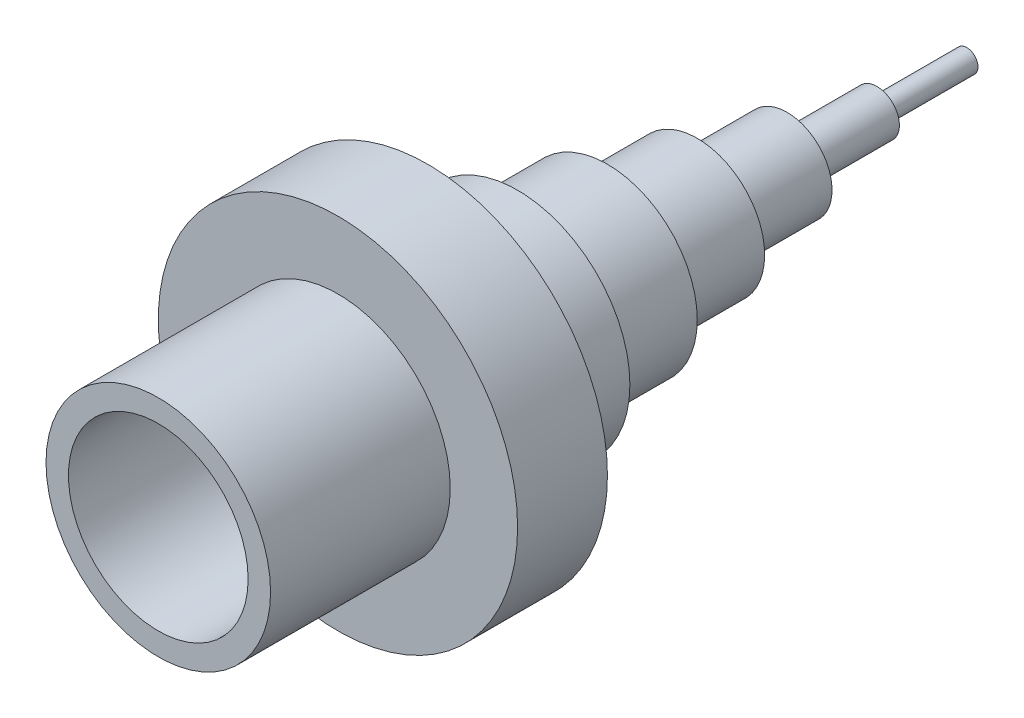
ISO-10303-21;
HEADER;
FILE_DESCRIPTION(('STEP AP214'),'2;1');
FILE_NAME('part.step','',(''),(''),'','','');
FILE_SCHEMA(('AUTOMOTIVE_DESIGN { 1 0 10303 214 1 1 1 1 }'));
ENDSEC;
DATA;
#1=APPLICATION_CONTEXT('core data for automotive mechanical design processes');
#2=APPLICATION_PROTOCOL_DEFINITION('international standard','automotive_design',2000,#1);
#3=PRODUCT_CONTEXT('',#1,'mechanical');
#4=PRODUCT('Part','Part','',(#3));
#5=PRODUCT_RELATED_PRODUCT_CATEGORY('part','',(#4));
#6=PRODUCT_DEFINITION_FORMATION('','',#4);
#7=PRODUCT_DEFINITION_CONTEXT('part definition',#1,'design');
#8=PRODUCT_DEFINITION('design','',#6,#7);
#9=PRODUCT_DEFINITION_SHAPE('','',#8);
#10=(LENGTH_UNIT() NAMED_UNIT(*) SI_UNIT(.MILLI.,.METRE.));
#11=(NAMED_UNIT(*) PLANE_ANGLE_UNIT() SI_UNIT($,.RADIAN.));
#12=(NAMED_UNIT(*) SI_UNIT($,.STERADIAN.) SOLID_ANGLE_UNIT());
#13=UNCERTAINTY_MEASURE_WITH_UNIT(LENGTH_MEASURE(1.E-05),#10,'distance_accuracy_value','');
#14=(GEOMETRIC_REPRESENTATION_CONTEXT(3) GLOBAL_UNCERTAINTY_ASSIGNED_CONTEXT((#13)) GLOBAL_UNIT_ASSIGNED_CONTEXT((#10,
#11,#12)) REPRESENTATION_CONTEXT('',''));
#15=CARTESIAN_POINT('',(0.,0.,0.));
#16=DIRECTION('',(0.,0.,1.));
#17=DIRECTION('',(1.,0.,0.));
#18=AXIS2_PLACEMENT_3D('',#15,#16,#17);
#19=CARTESIAN_POINT('',(0.,0.,-20.));
#20=DIRECTION('',(0.,0.,1.));
#21=DIRECTION('',(1.,0.,0.));
#22=AXIS2_PLACEMENT_3D('',#19,#20,#21);
#23=CYLINDRICAL_SURFACE('',#22,40.);
#24=CARTESIAN_POINT('',(0.,0.,-20.));
#25=DIRECTION('',(0.,0.,1.));
#26=DIRECTION('',(1.,0.,0.));
#27=AXIS2_PLACEMENT_3D('',#24,#25,#26);
#28=CIRCLE('',#27,40.);
#29=CARTESIAN_POINT('',(40.,0.,-20.));
#30=VERTEX_POINT('',#29);
#31=EDGE_CURVE('E42',#30,#30,#28,.T.);
#32=ORIENTED_EDGE('',*,*,#31,.T.);
#33=EDGE_LOOP('',(#32));
#34=FACE_BOUND('',#33,.T.);
#35=CARTESIAN_POINT('',(0.,0.,0.));
#36=DIRECTION('',(0.,0.,1.));
#37=DIRECTION('',(1.,0.,0.));
#38=AXIS2_PLACEMENT_3D('',#35,#36,#37);
#39=CIRCLE('',#38,40.);
#40=CARTESIAN_POINT('',(40.,0.,0.));
#41=VERTEX_POINT('',#40);
#42=EDGE_CURVE('E47',#41,#41,#39,.T.);
#43=ORIENTED_EDGE('',*,*,#42,.F.);
#44=EDGE_LOOP('',(#43));
#45=FACE_BOUND('',#44,.T.);
#46=ADVANCED_FACE('F40',(#34,#45),#23,.T.);
#47=CARTESIAN_POINT('',(0.,0.,-20.));
#48=DIRECTION('',(0.,0.,1.));
#49=DIRECTION('',(1.,0.,0.));
#50=AXIS2_PLACEMENT_3D('',#47,#48,#49);
#51=PLANE('',#50);
#52=CARTESIAN_POINT('',(0.,0.,-20.));
#53=DIRECTION('',(0.,0.,1.));
#54=DIRECTION('',(1.,0.,0.));
#55=AXIS2_PLACEMENT_3D('',#52,#53,#54);
#56=CIRCLE('',#55,25.);
#57=CARTESIAN_POINT('',(25.,0.,-20.));
#58=VERTEX_POINT('',#57);
#59=EDGE_CURVE('E80',#58,#58,#56,.T.);
#60=ORIENTED_EDGE('',*,*,#59,.T.);
#61=EDGE_LOOP('',(#60));
#62=FACE_BOUND('',#61,.T.);
#63=ORIENTED_EDGE('',*,*,#31,.F.);
#64=EDGE_LOOP('',(#63));
#65=FACE_BOUND('',#64,.T.);
#66=ADVANCED_FACE('F108',(#62,#65),#51,.F.);
#67=CARTESIAN_POINT('',(0.,0.,0.));
#68=DIRECTION('',(0.,0.,1.));
#69=DIRECTION('',(1.,0.,0.));
#70=AXIS2_PLACEMENT_3D('',#67,#68,#69);
#71=PLANE('',#70);
#72=CARTESIAN_POINT('',(0.,0.,0.));
#73=DIRECTION('',(0.,0.,1.));
#74=DIRECTION('',(1.,0.,0.));
#75=AXIS2_PLACEMENT_3D('',#72,#73,#74);
#76=CIRCLE('',#75,25.);
#77=CARTESIAN_POINT('',(25.,0.,0.));
#78=VERTEX_POINT('',#77);
#79=EDGE_CURVE('E10',#78,#78,#76,.T.);
#80=ORIENTED_EDGE('',*,*,#79,.F.);
#81=EDGE_LOOP('',(#80));
#82=FACE_BOUND('',#81,.T.);
#83=ORIENTED_EDGE('',*,*,#42,.T.);
#84=EDGE_LOOP('',(#83));
#85=FACE_BOUND('',#84,.T.);
#86=ADVANCED_FACE('F113',(#82,#85),#71,.T.);
#87=CARTESIAN_POINT('',(0.,0.,-40.));
#88=DIRECTION('',(0.,0.,1.));
#89=DIRECTION('',(1.,0.,0.));
#90=AXIS2_PLACEMENT_3D('',#87,#88,#89);
#91=CYLINDRICAL_SURFACE('',#90,25.);
#92=CARTESIAN_POINT('',(0.,0.,-40.));
#93=DIRECTION('',(0.,0.,1.));
#94=DIRECTION('',(1.,0.,0.));
#95=AXIS2_PLACEMENT_3D('',#92,#93,#94);
#96=CIRCLE('',#95,25.);
#97=CARTESIAN_POINT('',(25.,0.,-40.));
#98=VERTEX_POINT('',#97);
#99=EDGE_CURVE('E73',#98,#98,#96,.T.);
#100=ORIENTED_EDGE('',*,*,#99,.T.);
#101=EDGE_LOOP('',(#100));
#102=FACE_BOUND('',#101,.T.);
#103=ORIENTED_EDGE('',*,*,#59,.F.);
#104=EDGE_LOOP('',(#103));
#105=FACE_BOUND('',#104,.T.);
#106=ADVANCED_FACE('F122',(#102,#105),#91,.T.);
#107=CARTESIAN_POINT('',(0.,0.,-40.));
#108=DIRECTION('',(0.,0.,1.));
#109=DIRECTION('',(1.,0.,0.));
#110=AXIS2_PLACEMENT_3D('',#107,#108,#109);
#111=PLANE('',#110);
#112=CARTESIAN_POINT('',(0.,0.,-40.));
#113=DIRECTION('',(0.,0.,1.));
#114=DIRECTION('',(1.,0.,0.));
#115=AXIS2_PLACEMENT_3D('',#112,#113,#114);
#116=CIRCLE('',#115,20.);
#117=CARTESIAN_POINT('',(20.,0.,-40.));
#118=VERTEX_POINT('',#117);
#119=EDGE_CURVE('E75',#118,#118,#116,.T.);
#120=ORIENTED_EDGE('',*,*,#119,.T.);
#121=EDGE_LOOP('',(#120));
#122=FACE_BOUND('',#121,.T.);
#123=ORIENTED_EDGE('',*,*,#99,.F.);
#124=EDGE_LOOP('',(#123));
#125=FACE_BOUND('',#124,.T.);
#126=ADVANCED_FACE('F130',(#122,#125),#111,.F.);
#127=CARTESIAN_POINT('',(0.,0.,-60.));
#128=DIRECTION('',(0.,0.,1.));
#129=DIRECTION('',(1.,0.,0.));
#130=AXIS2_PLACEMENT_3D('',#127,#128,#129);
#131=CYLINDRICAL_SURFACE('',#130,20.);
#132=CARTESIAN_POINT('',(0.,0.,-60.));
#133=DIRECTION('',(0.,0.,1.));
#134=DIRECTION('',(1.,0.,0.));
#135=AXIS2_PLACEMENT_3D('',#132,#133,#134);
#136=CIRCLE('',#135,20.);
#137=CARTESIAN_POINT('',(20.,0.,-60.));
#138=VERTEX_POINT('',#137);
#139=EDGE_CURVE('E69',#138,#138,#136,.T.);
#140=ORIENTED_EDGE('',*,*,#139,.T.);
#141=EDGE_LOOP('',(#140));
#142=FACE_BOUND('',#141,.T.);
#143=ORIENTED_EDGE('',*,*,#119,.F.);
#144=EDGE_LOOP('',(#143));
#145=FACE_BOUND('',#144,.T.);
#146=ADVANCED_FACE('F132',(#142,#145),#131,.T.);
#147=CARTESIAN_POINT('',(0.,0.,-60.));
#148=DIRECTION('',(0.,0.,1.));
#149=DIRECTION('',(1.,0.,0.));
#150=AXIS2_PLACEMENT_3D('',#147,#148,#149);
#151=PLANE('',#150);
#152=CARTESIAN_POINT('',(0.,0.,-60.));
#153=DIRECTION('',(0.,0.,1.));
#154=DIRECTION('',(1.,0.,0.));
#155=AXIS2_PLACEMENT_3D('',#152,#153,#154);
#156=CIRCLE('',#155,15.);
#157=CARTESIAN_POINT('',(15.,0.,-60.));
#158=VERTEX_POINT('',#157);
#159=EDGE_CURVE('E67',#158,#158,#156,.T.);
#160=ORIENTED_EDGE('',*,*,#159,.T.);
#161=EDGE_LOOP('',(#160));
#162=FACE_BOUND('',#161,.T.);
#163=ORIENTED_EDGE('',*,*,#139,.F.);
#164=EDGE_LOOP('',(#163));
#165=FACE_BOUND('',#164,.T.);
#166=ADVANCED_FACE('F140',(#162,#165),#151,.F.);
#167=CARTESIAN_POINT('',(0.,0.,-80.));
#168=DIRECTION('',(0.,0.,1.));
#169=DIRECTION('',(1.,0.,0.));
#170=AXIS2_PLACEMENT_3D('',#167,#168,#169);
#171=CYLINDRICAL_SURFACE('',#170,15.);
#172=CARTESIAN_POINT('',(0.,0.,-80.));
#173=DIRECTION('',(0.,0.,1.));
#174=DIRECTION('',(1.,0.,0.));
#175=AXIS2_PLACEMENT_3D('',#172,#173,#174);
#176=CIRCLE('',#175,15.);
#177=CARTESIAN_POINT('',(15.,0.,-80.));
#178=VERTEX_POINT('',#177);
#179=EDGE_CURVE('E68',#178,#178,#176,.T.);
#180=ORIENTED_EDGE('',*,*,#179,.T.);
#181=EDGE_LOOP('',(#180));
#182=FACE_BOUND('',#181,.T.);
#183=ORIENTED_EDGE('',*,*,#159,.F.);
#184=EDGE_LOOP('',(#183));
#185=FACE_BOUND('',#184,.T.);
#186=ADVANCED_FACE('F145',(#182,#185),#171,.T.);
#187=CARTESIAN_POINT('',(0.,0.,-80.));
#188=DIRECTION('',(0.,0.,1.));
#189=DIRECTION('',(1.,0.,0.));
#190=AXIS2_PLACEMENT_3D('',#187,#188,#189);
#191=PLANE('',#190);
#192=CARTESIAN_POINT('',(0.,0.,-80.));
#193=DIRECTION('',(0.,0.,1.));
#194=DIRECTION('',(1.,0.,0.));
#195=AXIS2_PLACEMENT_3D('',#192,#193,#194);
#196=CIRCLE('',#195,10.);
#197=CARTESIAN_POINT('',(10.,0.,-80.));
#198=VERTEX_POINT('',#197);
#199=EDGE_CURVE('E62',#198,#198,#196,.T.);
#200=ORIENTED_EDGE('',*,*,#199,.T.);
#201=EDGE_LOOP('',(#200));
#202=FACE_BOUND('',#201,.T.);
#203=ORIENTED_EDGE('',*,*,#179,.F.);
#204=EDGE_LOOP('',(#203));
#205=FACE_BOUND('',#204,.T.);
#206=ADVANCED_FACE('F149',(#202,#205),#191,.F.);
#207=CARTESIAN_POINT('',(0.,0.,-100.));
#208=DIRECTION('',(0.,0.,1.));
#209=DIRECTION('',(1.,0.,0.));
#210=AXIS2_PLACEMENT_3D('',#207,#208,#209);
#211=CYLINDRICAL_SURFACE('',#210,10.);
#212=CARTESIAN_POINT('',(0.,0.,-100.));
#213=DIRECTION('',(0.,0.,1.));
#214=DIRECTION('',(1.,0.,0.));
#215=AXIS2_PLACEMENT_3D('',#212,#213,#214);
#216=CIRCLE('',#215,10.);
#217=CARTESIAN_POINT('',(10.,0.,-100.));
#218=VERTEX_POINT('',#217);
#219=EDGE_CURVE('E61',#218,#218,#216,.T.);
#220=ORIENTED_EDGE('',*,*,#219,.T.);
#221=EDGE_LOOP('',(#220));
#222=FACE_BOUND('',#221,.T.);
#223=ORIENTED_EDGE('',*,*,#199,.F.);
#224=EDGE_LOOP('',(#223));
#225=FACE_BOUND('',#224,.T.);
#226=ADVANCED_FACE('F102',(#222,#225),#211,.T.);
#227=CARTESIAN_POINT('',(0.,0.,-100.));
#228=DIRECTION('',(0.,0.,1.));
#229=DIRECTION('',(1.,0.,0.));
#230=AXIS2_PLACEMENT_3D('',#227,#228,#229);
#231=PLANE('',#230);
#232=CARTESIAN_POINT('',(0.,0.,-100.));
#233=DIRECTION('',(0.,0.,1.));
#234=DIRECTION('',(1.,0.,0.));
#235=AXIS2_PLACEMENT_3D('',#232,#233,#234);
#236=CIRCLE('',#235,5.);
#237=CARTESIAN_POINT('',(5.,0.,-100.));
#238=VERTEX_POINT('',#237);
#239=EDGE_CURVE('E64',#238,#238,#236,.T.);
#240=ORIENTED_EDGE('',*,*,#239,.T.);
#241=EDGE_LOOP('',(#240));
#242=FACE_BOUND('',#241,.T.);
#243=ORIENTED_EDGE('',*,*,#219,.F.);
#244=EDGE_LOOP('',(#243));
#245=FACE_BOUND('',#244,.T.);
#246=ADVANCED_FACE('F89',(#242,#245),#231,.F.);
#247=CARTESIAN_POINT('',(0.,0.,-120.));
#248=DIRECTION('',(0.,0.,1.));
#249=DIRECTION('',(1.,0.,0.));
#250=AXIS2_PLACEMENT_3D('',#247,#248,#249);
#251=CYLINDRICAL_SURFACE('',#250,5.);
#252=CARTESIAN_POINT('',(0.,0.,-120.));
#253=DIRECTION('',(0.,0.,1.));
#254=DIRECTION('',(1.,0.,0.));
#255=AXIS2_PLACEMENT_3D('',#252,#253,#254);
#256=CIRCLE('',#255,5.);
#257=CARTESIAN_POINT('',(5.,0.,-120.));
#258=VERTEX_POINT('',#257);
#259=EDGE_CURVE('E59',#258,#258,#256,.T.);
#260=ORIENTED_EDGE('',*,*,#259,.T.);
#261=EDGE_LOOP('',(#260));
#262=FACE_BOUND('',#261,.T.);
#263=ORIENTED_EDGE('',*,*,#239,.F.);
#264=EDGE_LOOP('',(#263));
#265=FACE_BOUND('',#264,.T.);
#266=ADVANCED_FACE('F95',(#262,#265),#251,.T.);
#267=CARTESIAN_POINT('',(0.,0.,-120.));
#268=DIRECTION('',(0.,0.,1.));
#269=DIRECTION('',(1.,0.,0.));
#270=AXIS2_PLACEMENT_3D('',#267,#268,#269);
#271=PLANE('',#270);
#272=CARTESIAN_POINT('',(0.,0.,-120.));
#273=DIRECTION('',(0.,0.,1.));
#274=DIRECTION('',(1.,0.,0.));
#275=AXIS2_PLACEMENT_3D('',#272,#273,#274);
#276=CIRCLE('',#275,2.5);
#277=CARTESIAN_POINT('',(2.5,0.,-120.));
#278=VERTEX_POINT('',#277);
#279=EDGE_CURVE('E37',#278,#278,#276,.T.);
#280=ORIENTED_EDGE('',*,*,#279,.T.);
#281=EDGE_LOOP('',(#280));
#282=FACE_BOUND('',#281,.T.);
#283=ORIENTED_EDGE('',*,*,#259,.F.);
#284=EDGE_LOOP('',(#283));
#285=FACE_BOUND('',#284,.T.);
#286=ADVANCED_FACE('F92',(#282,#285),#271,.F.);
#287=CARTESIAN_POINT('',(0.,0.,-140.));
#288=DIRECTION('',(0.,0.,1.));
#289=DIRECTION('',(1.,0.,0.));
#290=AXIS2_PLACEMENT_3D('',#287,#288,#289);
#291=CYLINDRICAL_SURFACE('',#290,2.5);
#292=CARTESIAN_POINT('',(0.,0.,-140.));
#293=DIRECTION('',(0.,0.,1.));
#294=DIRECTION('',(1.,0.,0.));
#295=AXIS2_PLACEMENT_3D('',#292,#293,#294);
#296=CIRCLE('',#295,2.5);
#297=CARTESIAN_POINT('',(2.5,0.,-140.));
#298=VERTEX_POINT('',#297);
#299=EDGE_CURVE('E54',#298,#298,#296,.T.);
#300=ORIENTED_EDGE('',*,*,#299,.T.);
#301=EDGE_LOOP('',(#300));
#302=FACE_BOUND('',#301,.T.);
#303=ORIENTED_EDGE('',*,*,#279,.F.);
#304=EDGE_LOOP('',(#303));
#305=FACE_BOUND('',#304,.T.);
#306=ADVANCED_FACE('F105',(#302,#305),#291,.T.);
#307=CARTESIAN_POINT('',(0.,0.,-140.));
#308=DIRECTION('',(0.,0.,1.));
#309=DIRECTION('',(1.,0.,0.));
#310=AXIS2_PLACEMENT_3D('',#307,#308,#309);
#311=PLANE('',#310);
#312=CARTESIAN_POINT('',(0.,0.,-140.));
#313=DIRECTION('',(0.,0.,1.));
#314=DIRECTION('',(1.,0.,0.));
#315=AXIS2_PLACEMENT_3D('',#312,#313,#314);
#316=CIRCLE('',#315,1.5);
#317=CARTESIAN_POINT('',(1.5,0.,-140.));
#318=VERTEX_POINT('',#317);
#319=EDGE_CURVE('E265',#318,#318,#316,.T.);
#320=ORIENTED_EDGE('',*,*,#319,.T.);
#321=EDGE_LOOP('',(#320));
#322=FACE_BOUND('',#321,.T.);
#323=ORIENTED_EDGE('',*,*,#299,.F.);
#324=EDGE_LOOP('',(#323));
#325=FACE_BOUND('',#324,.T.);
#326=ADVANCED_FACE('F200',(#322,#325),#311,.F.);
#327=CARTESIAN_POINT('',(0.,0.,40.));
#328=DIRECTION('',(0.,0.,-1.));
#329=DIRECTION('',(-1.,0.,0.));
#330=AXIS2_PLACEMENT_3D('',#327,#328,#329);
#331=CYLINDRICAL_SURFACE('',#330,25.);
#332=CARTESIAN_POINT('',(0.,0.,40.));
#333=DIRECTION('',(0.,0.,1.));
#334=DIRECTION('',(1.,0.,0.));
#335=AXIS2_PLACEMENT_3D('',#332,#333,#334);
#336=CIRCLE('',#335,25.);
#337=CARTESIAN_POINT('',(25.,0.,40.));
#338=VERTEX_POINT('',#337);
#339=EDGE_CURVE('E52',#338,#338,#336,.T.);
#340=ORIENTED_EDGE('',*,*,#339,.F.);
#341=EDGE_LOOP('',(#340));
#342=FACE_BOUND('',#341,.T.);
#343=ORIENTED_EDGE('',*,*,#79,.T.);
#344=EDGE_LOOP('',(#343));
#345=FACE_BOUND('',#344,.T.);
#346=ADVANCED_FACE('F210',(#342,#345),#331,.T.);
#347=CARTESIAN_POINT('',(0.,0.,40.));
#348=DIRECTION('',(0.,0.,1.));
#349=DIRECTION('',(1.,0.,0.));
#350=AXIS2_PLACEMENT_3D('',#347,#348,#349);
#351=PLANE('',#350);
#352=CARTESIAN_POINT('',(0.,0.,40.));
#353=DIRECTION('',(0.,0.,1.));
#354=DIRECTION('',(1.,0.,0.));
#355=AXIS2_PLACEMENT_3D('',#352,#353,#354);
#356=CIRCLE('',#355,20.);
#357=CARTESIAN_POINT('',(20.,0.,40.));
#358=VERTEX_POINT('',#357);
#359=EDGE_CURVE('E266',#358,#358,#356,.T.);
#360=ORIENTED_EDGE('',*,*,#359,.F.);
#361=EDGE_LOOP('',(#360));
#362=FACE_BOUND('',#361,.T.);
#363=ORIENTED_EDGE('',*,*,#339,.T.);
#364=EDGE_LOOP('',(#363));
#365=FACE_BOUND('',#364,.T.);
#366=ADVANCED_FACE('F216',(#362,#365),#351,.T.);
#367=CARTESIAN_POINT('',(0.,0.,0.));
#368=DIRECTION('',(0.,0.,1.));
#369=DIRECTION('',(1.,0.,0.));
#370=AXIS2_PLACEMENT_3D('',#367,#368,#369);
#371=CYLINDRICAL_SURFACE('',#370,20.);
#372=CARTESIAN_POINT('',(0.,0.,0.));
#373=DIRECTION('',(0.,0.,1.));
#374=DIRECTION('',(1.,0.,0.));
#375=AXIS2_PLACEMENT_3D('',#372,#373,#374);
#376=CIRCLE('',#375,20.);
#377=CARTESIAN_POINT('',(20.,0.,0.));
#378=VERTEX_POINT('',#377);
#379=EDGE_CURVE('E267',#378,#378,#376,.T.);
#380=ORIENTED_EDGE('',*,*,#379,.F.);
#381=EDGE_LOOP('',(#380));
#382=FACE_BOUND('',#381,.T.);
#383=ORIENTED_EDGE('',*,*,#359,.T.);
#384=EDGE_LOOP('',(#383));
#385=FACE_BOUND('',#384,.T.);
#386=ADVANCED_FACE('F226',(#382,#385),#371,.F.);
#387=CARTESIAN_POINT('',(0.,0.,0.));
#388=DIRECTION('',(0.,0.,1.));
#389=DIRECTION('',(1.,0.,0.));
#390=AXIS2_PLACEMENT_3D('',#387,#388,#389);
#391=PLANE('',#390);
#392=CARTESIAN_POINT('',(0.,0.,0.));
#393=DIRECTION('',(0.,0.,1.));
#394=DIRECTION('',(1.,0.,0.));
#395=AXIS2_PLACEMENT_3D('',#392,#393,#394);
#396=CIRCLE('',#395,1.5);
#397=CARTESIAN_POINT('',(1.5,0.,0.));
#398=VERTEX_POINT('',#397);
#399=EDGE_CURVE('E264',#398,#398,#396,.T.);
#400=ORIENTED_EDGE('',*,*,#399,.F.);
#401=EDGE_LOOP('',(#400));
#402=FACE_BOUND('',#401,.T.);
#403=ORIENTED_EDGE('',*,*,#379,.T.);
#404=EDGE_LOOP('',(#403));
#405=FACE_BOUND('',#404,.T.);
#406=ADVANCED_FACE('F240',(#402,#405),#391,.T.);
#407=CARTESIAN_POINT('',(0.,0.,-140.));
#408=DIRECTION('',(0.,0.,1.));
#409=DIRECTION('',(1.,0.,0.));
#410=AXIS2_PLACEMENT_3D('',#407,#408,#409);
#411=CYLINDRICAL_SURFACE('',#410,1.5);
#412=ORIENTED_EDGE('',*,*,#319,.F.);
#413=EDGE_LOOP('',(#412));
#414=FACE_BOUND('',#413,.T.);
#415=ORIENTED_EDGE('',*,*,#399,.T.);
#416=EDGE_LOOP('',(#415));
#417=FACE_BOUND('',#416,.T.);
#418=ADVANCED_FACE('F246',(#414,#417),#411,.F.);
#419=CLOSED_SHELL('',(#46,#66,#86,#106,#126,#146,#166,#186,#206,#226,#246,#266,#286,#306,#326,
#346,#366,#386,#406,#418));
#420=MANIFOLD_SOLID_BREP('B2',#419);
#421=ADVANCED_BREP_SHAPE_REPRESENTATION('',(#18,#420),#14);
#422=SHAPE_DEFINITION_REPRESENTATION(#9,#421);
ENDSEC;
END-ISO-10303-21;
